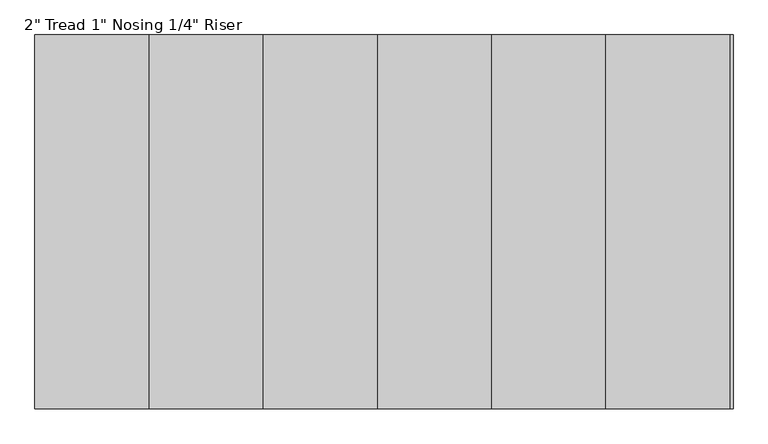
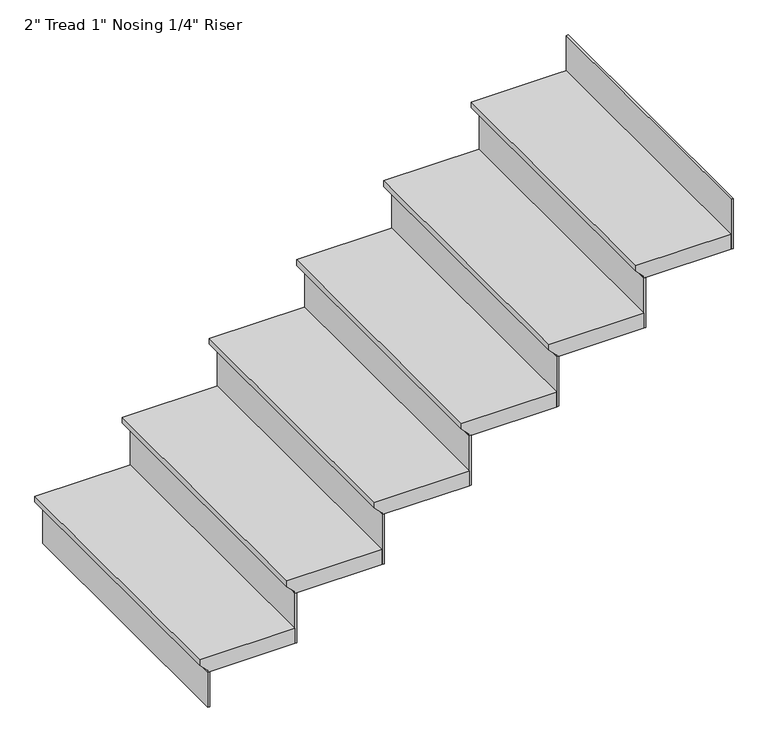
"""IFC4 building model written with IfcOpenShell, lengths in millimetres: stair flight geometry."""

from ifc_helpers import new_model, si_unit, origin, place, context, project, spatial, faceted_brep, source, transform, mapped, element, save


def stair_flight_290ad292(model_context):
    return source(origin(), model_context, "Body", "Brep", [
        faceted_brep([(-9231.9118598, 4340.1368529, 150.2833333), (-9231.9118598, 4340.1368529, 169.3333333), (-9231.9118598, 5254.5368529, 169.3333333), (-9231.9118598, 5254.5368529, 150.2833333), (-9206.5118598, 4340.1368529, 124.8833333), (-9206.5118598, 5254.5368529, 124.8833333), (-8927.1118598, 4340.1368529, 169.3333333), (-8927.1118598, 5254.5368529, 169.3333333), (-9206.5118598, 5254.5368529, 118.5333333), (-8927.1118598, 5254.5368529, 118.5333333), (-8927.1118598, 4340.1368529, 118.5333333), (-9206.5118598, 4340.1368529, 118.5333333)], [[[0, 1, 2, 3]], [[4, 0, 3, 5]], [[2, 1, 6, 7]], [[8, 9, 10, 11]], [[2, 7, 9, 8, 5, 3]], [[8, 11, 4, 5]], [[6, 1, 0, 4, 11, 10]], [[7, 6, 10, 9]]]),
        faceted_brep([(-9206.5118598, 4340.1368529, 118.5333333), (-9206.5118598, 4340.1368529, 0.0), (-9200.1618598, 4340.1368529, 0.0), (-9200.1618598, 4340.1368529, 118.5333333), (-9206.5118598, 5254.5368529, 118.5333333), (-9200.1618598, 5254.5368529, 118.5333333), (-9200.1618598, 5254.5368529, 0.0), (-9206.5118598, 5254.5368529, 0.0)], [[[0, 1, 2, 3]], [[4, 5, 6, 7]], [[1, 0, 4, 7]], [[2, 1, 7, 6]], [[3, 2, 6, 5]], [[0, 3, 5, 4]]]),
        faceted_brep([(-8927.1118598, 4340.1368529, 287.8666667), (-8927.1118598, 4340.1368529, 118.5333333), (-8920.7618598, 4340.1368529, 118.5333333), (-8920.7618598, 4340.1368529, 287.8666667), (-8927.1118598, 5254.5368529, 287.8666667), (-8920.7618598, 5254.5368529, 287.8666667), (-8920.7618598, 5254.5368529, 118.5333333), (-8927.1118598, 5254.5368529, 118.5333333)], [[[0, 1, 2, 3]], [[4, 5, 6, 7]], [[1, 0, 4, 7]], [[2, 1, 7, 6]], [[3, 2, 6, 5]], [[0, 3, 5, 4]]]),
        faceted_brep([(-8952.5118598, 5254.5368529, 338.6666667), (-8952.5118598, 4340.1368529, 338.6666667), (-8647.7118598, 4340.1368529, 338.6666667), (-8647.7118598, 5254.5368529, 338.6666667), (-8927.1118598, 5254.5368529, 287.8666667), (-8647.7118598, 5254.5368529, 287.8666667), (-8647.7118598, 4340.1368529, 287.8666667), (-8927.1118598, 4340.1368529, 287.8666667), (-8927.1118598, 5254.5368529, 294.2166667), (-8952.5118598, 5254.5368529, 319.6166667), (-8927.1118598, 4340.1368529, 294.2166667), (-8952.5118598, 4340.1368529, 319.6166667)], [[[0, 1, 2, 3]], [[4, 5, 6, 7]], [[0, 3, 5, 4, 8, 9]], [[4, 7, 10, 8]], [[2, 1, 11, 10, 7, 6]], [[3, 2, 6, 5]], [[11, 1, 0, 9]], [[10, 11, 9, 8]]]),
        faceted_brep([(-8647.7118598, 4340.1368529, 457.2), (-8647.7118598, 4340.1368529, 287.8666667), (-8641.3618598, 4340.1368529, 287.8666667), (-8641.3618598, 4340.1368529, 457.2), (-8647.7118598, 5254.5368529, 457.2), (-8641.3618598, 5254.5368529, 457.2), (-8641.3618598, 5254.5368529, 287.8666667), (-8647.7118598, 5254.5368529, 287.8666667)], [[[0, 1, 2, 3]], [[4, 5, 6, 7]], [[1, 0, 4, 7]], [[2, 1, 7, 6]], [[3, 2, 6, 5]], [[0, 3, 5, 4]]]),
        faceted_brep([(-8673.1118598, 5254.5368529, 508.0), (-8673.1118598, 4340.1368529, 508.0), (-8368.3118598, 4340.1368529, 508.0), (-8368.3118598, 5254.5368529, 508.0), (-8647.7118598, 5254.5368529, 457.2), (-8368.3118598, 5254.5368529, 457.2), (-8368.3118598, 4340.1368529, 457.2), (-8647.7118598, 4340.1368529, 457.2), (-8647.7118598, 5254.5368529, 463.55), (-8673.1118598, 5254.5368529, 488.95), (-8647.7118598, 4340.1368529, 463.55), (-8673.1118598, 4340.1368529, 488.95)], [[[0, 1, 2, 3]], [[4, 5, 6, 7]], [[0, 3, 5, 4, 8, 9]], [[4, 7, 10, 8]], [[2, 1, 11, 10, 7, 6]], [[3, 2, 6, 5]], [[11, 1, 0, 9]], [[10, 11, 9, 8]]]),
        faceted_brep([(-8368.3118598, 4340.1368529, 626.5333333), (-8368.3118598, 4340.1368529, 457.2), (-8361.9618598, 4340.1368529, 457.2), (-8361.9618598, 4340.1368529, 626.5333333), (-8368.3118598, 5254.5368529, 626.5333333), (-8361.9618598, 5254.5368529, 626.5333333), (-8361.9618598, 5254.5368529, 457.2), (-8368.3118598, 5254.5368529, 457.2)], [[[0, 1, 2, 3]], [[4, 5, 6, 7]], [[1, 0, 4, 7]], [[2, 1, 7, 6]], [[3, 2, 6, 5]], [[0, 3, 5, 4]]]),
        faceted_brep([(-8393.7118598, 5254.5368529, 677.3333333), (-8393.7118598, 4340.1368529, 677.3333333), (-8088.9118598, 4340.1368529, 677.3333333), (-8088.9118598, 5254.5368529, 677.3333333), (-8368.3118598, 5254.5368529, 626.5333333), (-8088.9118598, 5254.5368529, 626.5333333), (-8088.9118598, 4340.1368529, 626.5333333), (-8368.3118598, 4340.1368529, 626.5333333), (-8368.3118598, 5254.5368529, 632.8833333), (-8393.7118598, 5254.5368529, 658.2833333), (-8368.3118598, 4340.1368529, 632.8833333), (-8393.7118598, 4340.1368529, 658.2833333)], [[[0, 1, 2, 3]], [[4, 5, 6, 7]], [[0, 3, 5, 4, 8, 9]], [[4, 7, 10, 8]], [[2, 1, 11, 10, 7, 6]], [[3, 2, 6, 5]], [[11, 1, 0, 9]], [[10, 11, 9, 8]]]),
        faceted_brep([(-8088.9118598, 4340.1368529, 795.8666667), (-8088.9118598, 4340.1368529, 626.5333333), (-8082.5618598, 4340.1368529, 626.5333333), (-8082.5618598, 4340.1368529, 795.8666667), (-8088.9118598, 5254.5368529, 795.8666667), (-8082.5618598, 5254.5368529, 795.8666667), (-8082.5618598, 5254.5368529, 626.5333333), (-8088.9118598, 5254.5368529, 626.5333333)], [[[0, 1, 2, 3]], [[4, 5, 6, 7]], [[1, 0, 4, 7]], [[2, 1, 7, 6]], [[3, 2, 6, 5]], [[0, 3, 5, 4]]]),
        faceted_brep([(-8114.3118598, 5254.5368529, 846.6666667), (-8114.3118598, 4340.1368529, 846.6666667), (-7809.5118598, 4340.1368529, 846.6666667), (-7809.5118598, 5254.5368529, 846.6666667), (-8088.9118598, 5254.5368529, 795.8666667), (-7809.5118598, 5254.5368529, 795.8666667), (-7809.5118598, 4340.1368529, 795.8666667), (-8088.9118598, 4340.1368529, 795.8666667), (-8088.9118598, 5254.5368529, 802.2166667), (-8114.3118598, 5254.5368529, 827.6166667), (-8088.9118598, 4340.1368529, 802.2166667), (-8114.3118598, 4340.1368529, 827.6166667)], [[[0, 1, 2, 3]], [[4, 5, 6, 7]], [[0, 3, 5, 4, 8, 9]], [[4, 7, 10, 8]], [[2, 1, 11, 10, 7, 6]], [[3, 2, 6, 5]], [[11, 1, 0, 9]], [[10, 11, 9, 8]]]),
        faceted_brep([(-7530.1118598, 4340.1368529, 1134.5333333), (-7530.1118598, 4340.1368529, 965.2), (-7523.7618598, 4340.1368529, 965.2), (-7523.7618598, 4340.1368529, 1134.5333333), (-7530.1118598, 5254.5368529, 1134.5333333), (-7523.7618598, 5254.5368529, 1134.5333333), (-7523.7618598, 5254.5368529, 965.2), (-7530.1118598, 5254.5368529, 965.2)], [[[0, 1, 2, 3]], [[4, 5, 6, 7]], [[1, 0, 4, 7]], [[2, 1, 7, 6]], [[3, 2, 6, 5]], [[0, 3, 5, 4]]]),
        faceted_brep([(-7809.5118598, 4340.1368529, 965.2), (-7809.5118598, 4340.1368529, 795.8666667), (-7803.1618598, 4340.1368529, 795.8666667), (-7803.1618598, 4340.1368529, 965.2), (-7809.5118598, 5254.5368529, 965.2), (-7803.1618598, 5254.5368529, 965.2), (-7803.1618598, 5254.5368529, 795.8666667), (-7809.5118598, 5254.5368529, 795.8666667)], [[[0, 1, 2, 3]], [[4, 5, 6, 7]], [[1, 0, 4, 7]], [[2, 1, 7, 6]], [[3, 2, 6, 5]], [[0, 3, 5, 4]]]),
        faceted_brep([(-7530.1118598, 5254.5368529, 1016.0), (-7555.5118598, 5254.5368529, 1016.0), (-7834.9118598, 5254.5368529, 1016.0), (-7834.9118598, 4340.1368529, 1016.0), (-7530.1118598, 4340.1368529, 1016.0), (-7555.5118598, 5254.5368529, 965.2), (-7530.1118598, 5254.5368529, 965.2), (-7530.1118598, 4340.1368529, 965.2), (-7809.5118598, 4340.1368529, 965.2), (-7809.5118598, 5254.5368529, 965.2), (-7809.5118598, 5254.5368529, 971.55), (-7834.9118598, 5254.5368529, 996.95), (-7809.5118598, 4340.1368529, 971.55), (-7834.9118598, 4340.1368529, 996.95)], [[[0, 1, 2, 3, 4]], [[5, 6, 7, 8, 9]], [[1, 0, 6, 5]], [[2, 1, 5, 9, 10, 11]], [[9, 8, 12, 10]], [[4, 3, 13, 12, 8, 7]], [[0, 4, 7, 6]], [[13, 3, 2, 11]], [[12, 13, 11, 10]]]),
    ])


if __name__ == "__main__":
    model = new_model("IFC4")
    model_context = context("Model", 3, world=origin())
    ifc_project = project(units=[si_unit("LENGTHUNIT", "METRE", prefix="MILLI")], contexts=[model_context])
    site = spatial("IfcSite", under=ifc_project)
    building = spatial("IfcBuilding", under=site)
    placement = place(None, origin())
    stair_flight_shape = stair_flight_290ad292(model_context)
    element("IfcStairFlight", 1, ObjectType="2\" Tread 1\" Nosing 1/4\" Riser", at=placement, inside=building, context=model_context, shape_type="MappedRepresentation", body=[
        mapped(stair_flight_shape, transform((0.0, 0.0, 0.0), x_axis=(1.0, 0.0, 0.0), y_axis=(0.0, 1.0, 0.0), z_axis=(0.0, 0.0, 1.0))),
    ])
    save(model, "model.ifc")
